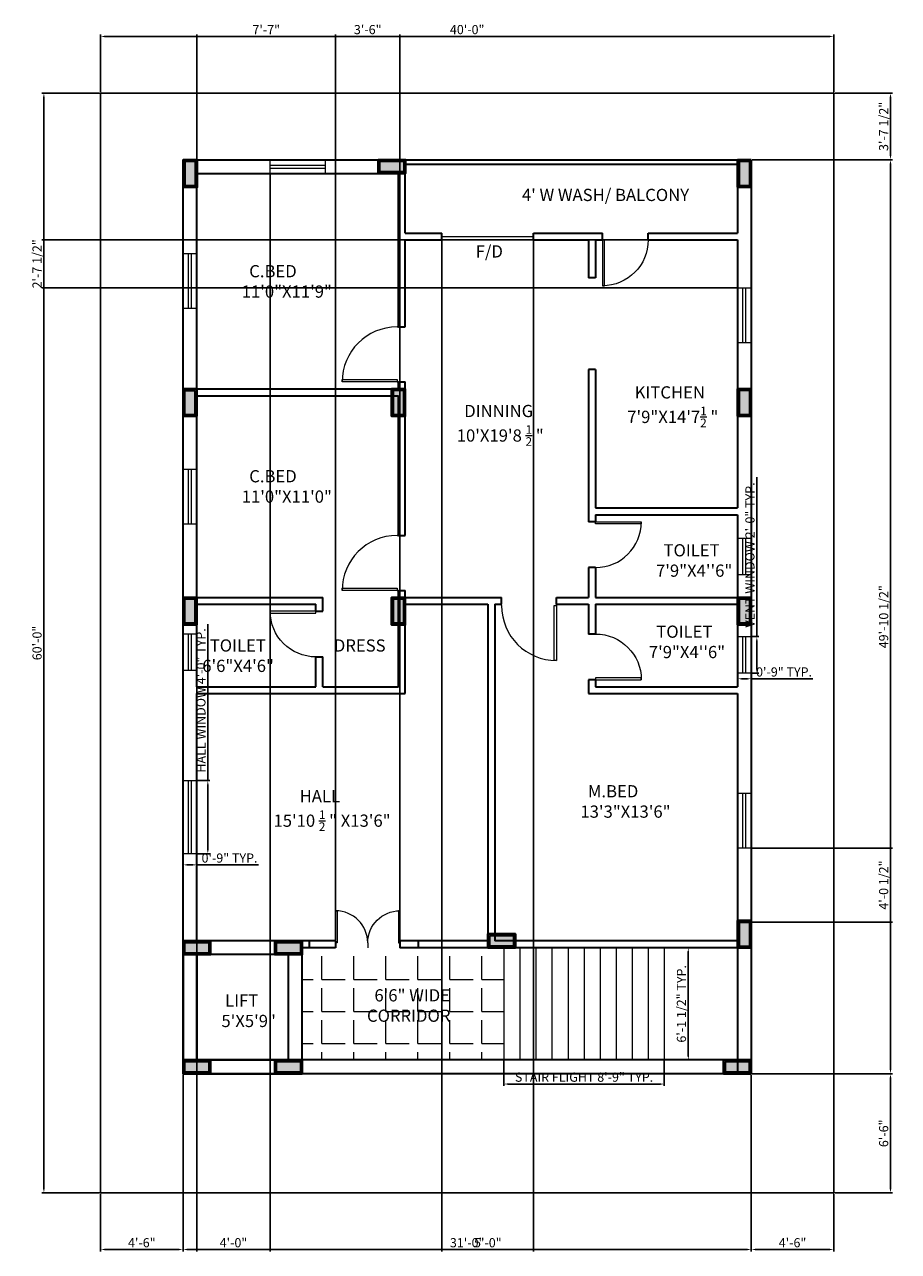
# Model space of a CAD drawing. Units: inches. Extents: x 1678 to 4856, y 4 to 3876.
# Tile 4 of 4: x 4284 to 4856, y 3070 to 3873. Entities that reach past the tile are written whole.
import ezdxf

# ---------------------------------------------------------------- set-up
doc = ezdxf.new("R2010")
doc.units = ezdxf.units.IN
for name, color, linetype, lineweight in [('A-ANNO-TEXT', 7, 'Continuous', 18), ('A-AREA-IDEN', 7, 'Continuous', 18), ('A-FLOR-EVTR', 7, 'Continuous', 35), ('A-FLOR-PATT', 252, 'Continuous', 13), ('COL', 6, 'Continuous', 40), ('compound wall', 7, 'Continuous', 30), ('DIMENSIONS', 6, 'Continuous', 18), ('doors', 2, 'Continuous', 18), ('stairs', 1, 'Continuous', 18), ('walls', 7, 'Continuous', 35), ('windows', 4, 'Continuous', 18)]:
    doc.layers.add(name, color=color, linetype=linetype, lineweight=lineweight)
doc.styles.get("Standard").update_dxf_attribs({"font": 'arial.ttf'})
doc.dimstyles.new('ISO-25', dxfattribs={"dimtxt": 6, "dimasz": 2.5, "dimexe": 1.25, "dimexo": 0.625, "dimtad": 1, "dimdec": 1, "dimlunit": 4, "dimtxsty": 'Standard', "dimcen": 2.5, "dimadec": 0, "dimazin": 0, "dimtfac": 1, "dimtdec": 1, "dimtmove": 0, "dimatfit": 3, "dimfxl": 1, "dimarcsym": 0})

# ---------------------------------------------------------------- blocks, each defined once
blk = doc.blocks.new('*U2')
for p, q in [((0, 0), (0, -6)), ((40, 0), (40, -6))]:
    blk.add_line(p, q)
blk.add_lwpolyline([(0, 0), (0, 40), (1.75, 40), (1.75, 0)], close=True)
blk.add_arc((0, 0), 40, 0, 90)
blk = doc.blocks.new('COLUMN-9x18')
h = blk.add_hatch(color=256)
h.dxf.hatch_style = 1
h.paths.add_polyline_path([(8, 1), (8, 17), (1, 17), (1, 1)])
for points in [[(9, 18), (9, 0), (0, 0), (0, 18)], [(8, 17), (8, 1), (1, 1), (1, 17)]]:
    blk.add_lwpolyline(points, close=True)
blk = doc.blocks.new('WIN-36')
for p, q in [((3.5, 0), (3.5, 36)), ((5.5, 0), (5.5, 36))]:
    blk.add_line(p, q)
blk.add_lwpolyline([(0, 0), (0, 36), (9, 36), (9, 0)], close=True)
blk = doc.blocks.new('WIN-24')
for p, q in [((3.5, 0), (3.5, 24)), ((5.5, 0), (5.5, 24))]:
    blk.add_line(p, q)
blk.add_lwpolyline([(0, 0), (0, 24), (9, 24), (9, 0)], close=True)
blk = doc.blocks.new('WIN-48')
for p, q in [((3.5, 0), (3.5, 48)), ((5.5, 0), (5.5, 48))]:
    blk.add_line(p, q)
blk.add_lwpolyline([(0, 0), (0, 48), (9, 48), (9, 0)], close=True)
blk = doc.blocks.new('SITE-PERIMETER-40x60')
for p, q in [((0, 720), (480, 720)), ((0, 0), (0, 720)), ((480, 720), (480, 0)), ((480, 0), (0, 0))]:
    blk.add_line(p, q)
blk = doc.blocks.new('STAIR-FLIGHT-11-TREAD-LINES')
for p, q in [((0, 73.5), (0, 0)), ((10.5, 73.5), (10.5, 0)), ((21, 73.5), (21, 0)), ((31.5, 73.5), (31.5, 0)), ((42, 73.5), (42, 0)), ((52.5, 73.5), (52.5, 0)), ((63, 73.5), (63, 0)), ((73.5, 73.5), (73.5, 0)), ((84, 73.5), (84, 0)), ((94.5, 73.5), (94.5, 0)), ((105, 73.5), (105, 0))]:
    blk.add_line(p, q)
blk = doc.blocks.new('LIFT-SHAFT-60x69')
for p, q in [((9, 9), (9, 78)), ((69, 9), (9, 9))]:
    blk.add_line(p, q)
blk.add_lwpolyline([(78, 87), (78, 87), (0, 87), (0, 0), (78, 0), (78, 82.5)])
blk.add_lwpolyline([(9, 9), (69, 9), (69, 78), (9, 78)], close=True)
blk = doc.blocks.new('*D46')
at = {"layer": 'Defpoints', "color": 0, "transparency": 16777216}
for p in [(4598, 3195.28), (4703, 3195.28), (4703, 3179.53)]:
    blk.add_point(p, dxfattribs=at)
at = {"layer": 'DIMENSIONS', "color": 0, "lineweight": -2, "transparency": 16777216}
for p, q in [((4598, 3194.65), (4598, 3178.28)), ((4703, 3194.65), (4703, 3178.28)), ((4600.5, 3179.53), (4700.5, 3179.53))]:
    blk.add_line(p, q, dxfattribs=at)
at = {"layer": 'DIMENSIONS', "color": 0, "transparency": 16777216}
for points in [[(4600.5, 3179.94), (4600.5, 3179.11), (4598, 3179.53)], [(4700.5, 3179.94), (4700.5, 3179.11), (4703, 3179.53)]]:
    blk.add_solid(points, dxfattribs=at)
at = {"layer": 'DIMENSIONS', "color": 0, "transparency": 16777216, "insert": (4650.5, 3183.25), "char_height": 6, "attachment_point": 5}
blk.add_mtext('STAIR FLIGHT 8\'-9" TYP.', dxfattribs=at)
blk = doc.blocks.new('*D47')
at = {"layer": 'Defpoints', "color": 0, "transparency": 16777216}
for p in [(4703, 3268.78), (4718.75, 3268.78), (4703, 3195.28)]:
    blk.add_point(p, dxfattribs=at)
at = {"layer": 'DIMENSIONS', "color": 0, "lineweight": -2, "transparency": 16777216}
for p, q in [((4703.63, 3268.78), (4720, 3268.78)), ((4718.75, 3197.78), (4718.75, 3266.28)), ((4703.63, 3195.28), (4720, 3195.28))]:
    blk.add_line(p, q, dxfattribs=at)
at = {"layer": 'DIMENSIONS', "color": 0, "transparency": 16777216}
for points in [[(4718.34, 3266.28), (4719.17, 3266.28), (4718.75, 3268.78)], [(4718.34, 3197.78), (4719.17, 3197.78), (4718.75, 3195.28)]]:
    blk.add_solid(points, dxfattribs=at)
at = {"layer": 'DIMENSIONS', "color": 0, "transparency": 16777216, "insert": (4715.03, 3232.03), "char_height": 6, "attachment_point": 5, "rotation": 90}
blk.add_mtext('6\'-1 1/2" TYP.', dxfattribs=at)
blk = doc.blocks.new('*D50')
at = {"layer": 'Defpoints', "color": 0, "transparency": 16777216}
for p in [(4760, 3472.44), (4763.6, 3472.44), (4760, 3448.44)]:
    blk.add_point(p, dxfattribs=at)
at = {"layer": 'DIMENSIONS', "color": 0, "lineweight": -2, "transparency": 16777216}
for p, q in [((4763.6, 3472.44), (4763.6, 3576.86)), ((4760.63, 3472.44), (4764.85, 3472.44)), ((4763.6, 3450.94), (4763.6, 3469.94)), ((4760.63, 3448.44), (4764.85, 3448.44))]:
    blk.add_line(p, q, dxfattribs=at)
at = {"layer": 'DIMENSIONS', "color": 0, "transparency": 16777216}
for points in [[(4763.19, 3469.94), (4764.02, 3469.94), (4763.6, 3472.44)], [(4763.19, 3450.94), (4764.02, 3450.94), (4763.6, 3448.44)]]:
    blk.add_solid(points, dxfattribs=at)
at = {"layer": 'DIMENSIONS', "color": 0, "transparency": 16777216, "insert": (4759.88, 3525.9), "char_height": 6, "attachment_point": 5, "rotation": 90}
blk.add_mtext('VENT WINDOW 2\'-0" TYP.', dxfattribs=at)
blk = doc.blocks.new('*D51')
at = {"layer": 'Defpoints', "color": 0, "transparency": 16777216}
for p in [(4751, 3448.44), (4760, 3448.44), (4760, 3444.84)]:
    blk.add_point(p, dxfattribs=at)
at = {"layer": 'DIMENSIONS', "color": 0, "lineweight": -2, "transparency": 16777216}
for p, q in [((4751, 3447.82), (4751, 3443.59)), ((4760, 3447.82), (4760, 3443.59)), ((4753.5, 3444.84), (4757.5, 3444.84)), ((4760, 3444.84), (4800.33, 3444.84))]:
    blk.add_line(p, q, dxfattribs=at)
at = {"layer": 'DIMENSIONS', "color": 0, "transparency": 16777216}
for points in [[(4753.5, 3445.26), (4753.5, 3444.42), (4751, 3444.84)], [(4757.5, 3445.26), (4757.5, 3444.42), (4760, 3444.84)]]:
    blk.add_solid(points, dxfattribs=at)
at = {"layer": 'DIMENSIONS', "color": 0, "transparency": 16777216, "insert": (4781.42, 3448.53), "char_height": 6, "attachment_point": 5}
blk.add_mtext('0\'-9" TYP.', dxfattribs=at)
blk = doc.blocks.new('*D52')
at = {"layer": 'Defpoints', "color": 0, "transparency": 16777216}
for p in [(4397, 3378.22), (4404.2, 3378.22), (4397, 3330.22)]:
    blk.add_point(p, dxfattribs=at)
at = {"layer": 'DIMENSIONS', "color": 0, "lineweight": -2, "transparency": 16777216}
for p, q in [((4404.2, 3378.22), (4404.2, 3480.62)), ((4397.63, 3378.22), (4405.45, 3378.22)), ((4404.2, 3332.72), (4404.2, 3375.72)), ((4397.63, 3330.22), (4405.45, 3330.22))]:
    blk.add_line(p, q, dxfattribs=at)
at = {"layer": 'DIMENSIONS', "color": 0, "transparency": 16777216}
for points in [[(4403.79, 3375.72), (4404.62, 3375.72), (4404.2, 3378.22)], [(4403.79, 3332.72), (4404.62, 3332.72), (4404.2, 3330.22)]]:
    blk.add_solid(points, dxfattribs=at)
at = {"layer": 'DIMENSIONS', "color": 0, "transparency": 16777216, "insert": (4400.48, 3430.67), "char_height": 6, "attachment_point": 5, "rotation": 90}
blk.add_mtext('HALL WINDOW 4\'-0" TYP.', dxfattribs=at)
blk = doc.blocks.new('*D53')
at = {"layer": 'Defpoints', "color": 0, "transparency": 16777216}
for p in [(4388, 3330.22), (4397, 3330.22), (4397, 3323.02)]:
    blk.add_point(p, dxfattribs=at)
at = {"layer": 'DIMENSIONS', "color": 0, "lineweight": -2, "transparency": 16777216}
for p, q in [((4388, 3329.6), (4388, 3321.77)), ((4397, 3329.6), (4397, 3321.77)), ((4390.5, 3323.02), (4394.5, 3323.02)), ((4397, 3323.02), (4437.33, 3323.02))]:
    blk.add_line(p, q, dxfattribs=at)
at = {"layer": 'DIMENSIONS', "color": 0, "transparency": 16777216}
for points in [[(4390.5, 3323.44), (4390.5, 3322.6), (4388, 3323.02)], [(4394.5, 3323.44), (4394.5, 3322.6), (4397, 3323.02)]]:
    blk.add_solid(points, dxfattribs=at)
at = {"layer": 'DIMENSIONS', "color": 0, "transparency": 16777216, "insert": (4418.42, 3326.71), "char_height": 6, "attachment_point": 5}
blk.add_mtext('0\'-9" TYP.', dxfattribs=at)
blk = doc.blocks.new('*D62')
at = {"layer": 'Defpoints', "color": 0, "transparency": 16777216}
for p in [(4814, 3865.38), (4334, 3828.28), (4814, 3828.28)]:
    blk.add_point(p, dxfattribs=at)
at = {"layer": 'DIMENSIONS', "color": 0, "lineweight": -2, "transparency": 16777216}
for p, q in [((4334, 3828.9), (4334, 3866.63)), ((4336.5, 3865.38), (4811.5, 3865.38)), ((4814, 3828.9), (4814, 3866.63))]:
    blk.add_line(p, q, dxfattribs=at)
at = {"layer": 'DIMENSIONS', "color": 0, "transparency": 16777216}
for points in [[(4336.5, 3865.79), (4336.5, 3864.96), (4334, 3865.38)], [(4811.5, 3865.79), (4811.5, 3864.96), (4814, 3865.38)]]:
    blk.add_solid(points, dxfattribs=at)
at = {"layer": 'DIMENSIONS', "color": 0, "transparency": 16777216, "insert": (4574, 3869.07), "char_height": 6, "attachment_point": 5}
blk.add_mtext('40\'-0"', dxfattribs=at)
blk = doc.blocks.new('*D63')
at = {"layer": 'Defpoints', "color": 0, "transparency": 16777216}
for p in [(4296.9, 3828.28), (4334, 3828.28), (4334, 3108.28)]:
    blk.add_point(p, dxfattribs=at)
at = {"layer": 'DIMENSIONS', "color": 0, "lineweight": -2, "transparency": 16777216}
for p, q in [((4333.38, 3828.28), (4295.65, 3828.28)), ((4296.9, 3110.78), (4296.9, 3825.78)), ((4333.38, 3108.28), (4295.65, 3108.28))]:
    blk.add_line(p, q, dxfattribs=at)
at = {"layer": 'DIMENSIONS', "color": 0, "transparency": 16777216}
for points in [[(4296.49, 3825.78), (4297.32, 3825.78), (4296.9, 3828.28)], [(4296.49, 3110.78), (4297.32, 3110.78), (4296.9, 3108.28)]]:
    blk.add_solid(points, dxfattribs=at)
at = {"layer": 'DIMENSIONS', "color": 0, "transparency": 16777216, "insert": (4293.22, 3468.28), "char_height": 6, "attachment_point": 5, "rotation": 90}
blk.add_mtext('60\'-0"', dxfattribs=at)
blk = doc.blocks.new('*D64')
at = {"layer": 'Defpoints', "color": 0, "transparency": 16777216}
for p in [(4388, 3186.28), (4760, 3186.28), (4760, 3071.18)]:
    blk.add_point(p, dxfattribs=at)
at = {"layer": 'DIMENSIONS', "color": 0, "lineweight": -2, "transparency": 16777216}
for p, q in [((4388, 3185.65), (4388, 3069.93)), ((4760, 3185.65), (4760, 3069.93)), ((4390.5, 3071.18), (4757.5, 3071.18))]:
    blk.add_line(p, q, dxfattribs=at)
at = {"layer": 'DIMENSIONS', "color": 0, "transparency": 16777216}
for points in [[(4390.5, 3071.59), (4390.5, 3070.76), (4388, 3071.18)], [(4757.5, 3071.59), (4757.5, 3070.76), (4760, 3071.18)]]:
    blk.add_solid(points, dxfattribs=at)
at = {"layer": 'DIMENSIONS', "color": 0, "transparency": 16777216, "insert": (4574, 3074.87), "char_height": 6, "attachment_point": 5}
blk.add_mtext('31\'-0"', dxfattribs=at)
blk = doc.blocks.new('*D65')
at = {"layer": 'Defpoints', "color": 0, "transparency": 16777216}
for p in [(4760, 3784.66), (4851.1, 3784.66), (4760, 3186.28)]:
    blk.add_point(p, dxfattribs=at)
at = {"layer": 'DIMENSIONS', "color": 0, "lineweight": -2, "transparency": 16777216}
for p, q in [((4760.63, 3784.66), (4852.35, 3784.66)), ((4851.1, 3188.78), (4851.1, 3782.16)), ((4760.63, 3186.28), (4852.35, 3186.28))]:
    blk.add_line(p, q, dxfattribs=at)
at = {"layer": 'DIMENSIONS', "color": 0, "transparency": 16777216}
for points in [[(4850.69, 3782.16), (4851.52, 3782.16), (4851.1, 3784.66)], [(4850.69, 3188.78), (4851.52, 3188.78), (4851.1, 3186.28)]]:
    blk.add_solid(points, dxfattribs=at)
at = {"layer": 'DIMENSIONS', "color": 0, "transparency": 16777216, "insert": (4847.38, 3485.47), "char_height": 6, "attachment_point": 5, "rotation": 90}
blk.add_mtext('49\'-10 1/2"', dxfattribs=at)
blk = doc.blocks.new('*D66')
at = {"layer": 'Defpoints', "color": 0, "transparency": 16777216}
for p in [(4388, 3186.28), (4334, 3108.28), (4388, 3071.18)]:
    blk.add_point(p, dxfattribs=at)
at = {"layer": 'DIMENSIONS', "color": 0, "lineweight": -2, "transparency": 16777216}
for p, q in [((4388, 3185.65), (4388, 3069.93)), ((4334, 3107.65), (4334, 3069.93)), ((4336.5, 3071.18), (4385.5, 3071.18))]:
    blk.add_line(p, q, dxfattribs=at)
at = {"layer": 'DIMENSIONS', "color": 0, "transparency": 16777216}
for points in [[(4336.5, 3071.59), (4336.5, 3070.76), (4334, 3071.18)], [(4385.5, 3071.59), (4385.5, 3070.76), (4388, 3071.18)]]:
    blk.add_solid(points, dxfattribs=at)
at = {"layer": 'DIMENSIONS', "color": 0, "transparency": 16777216, "insert": (4361, 3074.87), "char_height": 6, "attachment_point": 5}
blk.add_mtext('4\'-6"', dxfattribs=at)
blk = doc.blocks.new('*D67')
at = {"layer": 'Defpoints', "color": 0, "transparency": 16777216}
for p in [(4760, 3186.28), (4814, 3108.28), (4851.1, 3108.28)]:
    blk.add_point(p, dxfattribs=at)
at = {"layer": 'DIMENSIONS', "color": 0, "lineweight": -2, "transparency": 16777216}
for p, q in [((4760.63, 3186.28), (4852.35, 3186.28)), ((4851.1, 3183.78), (4851.1, 3110.78)), ((4814.63, 3108.28), (4852.35, 3108.28))]:
    blk.add_line(p, q, dxfattribs=at)
at = {"layer": 'DIMENSIONS', "color": 0, "transparency": 16777216}
for points in [[(4850.69, 3183.78), (4851.52, 3183.78), (4851.1, 3186.28)], [(4850.69, 3110.78), (4851.52, 3110.78), (4851.1, 3108.28)]]:
    blk.add_solid(points, dxfattribs=at)
at = {"layer": 'DIMENSIONS', "color": 0, "transparency": 16777216, "insert": (4847.42, 3147.28), "char_height": 6, "attachment_point": 5, "rotation": 90}
blk.add_mtext('6\'-6"', dxfattribs=at)
blk = doc.blocks.new('*D68')
at = {"layer": 'Defpoints', "color": 0, "transparency": 16777216}
for p in [(4814, 3828.28), (4851.1, 3828.28), (4760, 3784.66)]:
    blk.add_point(p, dxfattribs=at)
at = {"layer": 'DIMENSIONS', "color": 0, "lineweight": -2, "transparency": 16777216}
for p, q in [((4814.63, 3828.28), (4852.35, 3828.28)), ((4851.1, 3787.16), (4851.1, 3825.78)), ((4760.63, 3784.66), (4852.35, 3784.66))]:
    blk.add_line(p, q, dxfattribs=at)
at = {"layer": 'DIMENSIONS', "color": 0, "transparency": 16777216}
for points in [[(4850.69, 3825.78), (4851.52, 3825.78), (4851.1, 3828.28)], [(4850.69, 3787.16), (4851.52, 3787.16), (4851.1, 3784.66)]]:
    blk.add_solid(points, dxfattribs=at)
at = {"layer": 'DIMENSIONS', "color": 0, "transparency": 16777216, "insert": (4847.38, 3806.47), "char_height": 6, "attachment_point": 5, "rotation": 90}
blk.add_mtext('3\'-7 1/2"', dxfattribs=at)
blk = doc.blocks.new('*D69')
at = {"layer": 'Defpoints', "color": 0, "transparency": 16777216}
for p in [(4760, 3186.28), (4814, 3108.28), (4814, 3071.18)]:
    blk.add_point(p, dxfattribs=at)
at = {"layer": 'DIMENSIONS', "color": 0, "lineweight": -2, "transparency": 16777216}
for p, q in [((4760, 3185.65), (4760, 3069.93)), ((4814, 3107.65), (4814, 3069.93)), ((4762.5, 3071.18), (4811.5, 3071.18))]:
    blk.add_line(p, q, dxfattribs=at)
at = {"layer": 'DIMENSIONS', "color": 0, "transparency": 16777216}
for points in [[(4762.5, 3071.59), (4762.5, 3070.76), (4760, 3071.18)], [(4811.5, 3071.59), (4811.5, 3070.76), (4814, 3071.18)]]:
    blk.add_solid(points, dxfattribs=at)
at = {"layer": 'DIMENSIONS', "color": 0, "transparency": 16777216, "insert": (4787, 3074.87), "char_height": 6, "attachment_point": 5}
blk.add_mtext('4\'-6"', dxfattribs=at)
blk = doc.blocks.new('*D70')
at = {"layer": 'Defpoints', "color": 0, "transparency": 16777216}
for p in [(4397, 3775.66), (4445, 3775.66), (4445, 3071.18)]:
    blk.add_point(p, dxfattribs=at)
at = {"layer": 'DIMENSIONS', "color": 0, "lineweight": -2, "transparency": 16777216}
for p, q in [((4397, 3775.04), (4397, 3069.93)), ((4445, 3775.04), (4445, 3069.93)), ((4399.5, 3071.18), (4442.5, 3071.18))]:
    blk.add_line(p, q, dxfattribs=at)
at = {"layer": 'DIMENSIONS', "color": 0, "transparency": 16777216}
for points in [[(4399.5, 3071.59), (4399.5, 3070.76), (4397, 3071.18)], [(4442.5, 3071.59), (4442.5, 3070.76), (4445, 3071.18)]]:
    blk.add_solid(points, dxfattribs=at)
at = {"layer": 'DIMENSIONS', "color": 0, "transparency": 16777216, "insert": (4421, 3074.87), "char_height": 6, "attachment_point": 5}
blk.add_mtext('4\'-0"', dxfattribs=at)
blk = doc.blocks.new('*D71')
at = {"layer": 'Defpoints', "color": 0, "transparency": 16777216}
for p in [(4557.5, 3736.66), (4617.5, 3736.66), (4617.5, 3071.18)]:
    blk.add_point(p, dxfattribs=at)
at = {"layer": 'DIMENSIONS', "color": 0, "lineweight": -2, "transparency": 16777216}
for p, q in [((4557.5, 3736.04), (4557.5, 3069.93)), ((4617.5, 3736.04), (4617.5, 3069.93)), ((4560, 3071.18), (4615, 3071.18))]:
    blk.add_line(p, q, dxfattribs=at)
at = {"layer": 'DIMENSIONS', "color": 0, "transparency": 16777216}
for points in [[(4560, 3071.59), (4560, 3070.76), (4557.5, 3071.18)], [(4615, 3071.59), (4615, 3070.76), (4617.5, 3071.18)]]:
    blk.add_solid(points, dxfattribs=at)
at = {"layer": 'DIMENSIONS', "color": 0, "transparency": 16777216, "insert": (4587.5, 3074.87), "char_height": 6, "attachment_point": 5}
blk.add_mtext('5\'-0"', dxfattribs=at)
blk = doc.blocks.new('*D72')
at = {"layer": 'Defpoints', "color": 0, "transparency": 16777216}
for p in [(4487.89, 3865.38), (4397, 3273.28), (4487.89, 3273.28)]:
    blk.add_point(p, dxfattribs=at)
at = {"layer": 'DIMENSIONS', "color": 0, "lineweight": -2, "transparency": 16777216}
for p, q in [((4397, 3273.9), (4397, 3866.63)), ((4399.5, 3865.38), (4485.39, 3865.38)), ((4487.89, 3273.9), (4487.89, 3866.63))]:
    blk.add_line(p, q, dxfattribs=at)
at = {"layer": 'DIMENSIONS', "color": 0, "transparency": 16777216}
for points in [[(4399.5, 3865.79), (4399.5, 3864.96), (4397, 3865.38)], [(4485.39, 3865.79), (4485.39, 3864.96), (4487.89, 3865.38)]]:
    blk.add_solid(points, dxfattribs=at)
at = {"layer": 'DIMENSIONS', "color": 0, "transparency": 16777216, "insert": (4442.45, 3869), "char_height": 6, "attachment_point": 5}
blk.add_mtext('7\'-7"', dxfattribs=at)
blk = doc.blocks.new('*D73')
at = {"layer": 'Defpoints', "color": 0, "transparency": 16777216}
for p in [(4529.89, 3865.38), (4487.89, 3273.28), (4529.89, 3273.28)]:
    blk.add_point(p, dxfattribs=at)
at = {"layer": 'DIMENSIONS', "color": 0, "lineweight": -2, "transparency": 16777216}
for p, q in [((4487.89, 3273.9), (4487.89, 3866.63)), ((4490.39, 3865.38), (4527.39, 3865.38)), ((4529.89, 3273.9), (4529.89, 3866.63))]:
    blk.add_line(p, q, dxfattribs=at)
at = {"layer": 'DIMENSIONS', "color": 0, "transparency": 16777216}
for points in [[(4490.39, 3865.79), (4490.39, 3864.96), (4487.89, 3865.38)], [(4527.39, 3865.79), (4527.39, 3864.96), (4529.89, 3865.38)]]:
    blk.add_solid(points, dxfattribs=at)
at = {"layer": 'DIMENSIONS', "color": 0, "transparency": 16777216, "insert": (4508.89, 3869.07), "char_height": 6, "attachment_point": 5}
blk.add_mtext('3\'-6"', dxfattribs=at)
blk = doc.blocks.new('*D80')
at = {"layer": 'Defpoints', "color": 0, "transparency": 16777216}
for p in [(4751, 3732.16), (4296.9, 3700.81), (4751, 3700.81)]:
    blk.add_point(p, dxfattribs=at)
at = {"layer": 'DIMENSIONS', "color": 0, "lineweight": -2, "transparency": 16777216}
for p, q in [((4750.38, 3732.16), (4295.65, 3732.16)), ((4296.9, 3729.66), (4296.9, 3703.31)), ((4750.38, 3700.81), (4295.65, 3700.81))]:
    blk.add_line(p, q, dxfattribs=at)
at = {"layer": 'DIMENSIONS', "color": 0, "transparency": 16777216}
for points in [[(4296.49, 3729.66), (4297.32, 3729.66), (4296.9, 3732.16)], [(4296.49, 3703.31), (4297.32, 3703.31), (4296.9, 3700.81)]]:
    blk.add_solid(points, dxfattribs=at)
at = {"layer": 'DIMENSIONS', "color": 0, "transparency": 16777216, "insert": (4293.18, 3716.49), "char_height": 6, "attachment_point": 5, "rotation": 90}
blk.add_mtext('2\'-7 1/2"', dxfattribs=at)
blk = doc.blocks.new('*D81')
at = {"layer": 'Defpoints', "color": 0, "transparency": 16777216}
for p in [(4760, 3333.97), (4759, 3285.61), (4851.1, 3285.61)]:
    blk.add_point(p, dxfattribs=at)
at = {"layer": 'DIMENSIONS', "color": 0, "lineweight": -2, "transparency": 16777216}
for p, q in [((4760.63, 3333.97), (4852.35, 3333.97)), ((4851.1, 3331.47), (4851.1, 3288.11)), ((4759.63, 3285.61), (4852.35, 3285.61))]:
    blk.add_line(p, q, dxfattribs=at)
at = {"layer": 'DIMENSIONS', "color": 0, "transparency": 16777216}
for points in [[(4850.69, 3331.47), (4851.52, 3331.47), (4851.1, 3333.97)], [(4850.69, 3288.11), (4851.52, 3288.11), (4851.1, 3285.61)]]:
    blk.add_solid(points, dxfattribs=at)
at = {"layer": 'DIMENSIONS', "color": 0, "transparency": 16777216, "insert": (4847.38, 3309.79), "char_height": 6, "attachment_point": 5, "rotation": 90}
blk.add_mtext('4\'-0 1/2"', dxfattribs=at)

msp = doc.modelspace()

# ---------------------------------------------------------------- hatches: boundary and pattern name
at = {"layer": 'A-FLOR-PATT'}
h = msp.add_hatch(dxfattribs=at)
h.set_pattern_fill('ANGLE', color=256, scale=3)
h.set_pattern_definition([(0, (2760.532, 0), (0, 20.955), [15.24, -5.715]), (90, (2760.532, 0), (-20.955, 1e-15), [15.24, -5.715])])
h.paths.add_polyline_path([(4598, 3268.78), (4466, 3268.78), (4466, 3195.28), (4598, 3195.28)])

# ---------------------------------------------------------------- linework, layer by layer
at = {"layer": 'doors'}
msp.add_line((4557.5, 3734.41), (4617.5, 3734.41), dxfattribs=at)
at = {"layer": 'walls'}
for p, q in [((4388, 3784.66), (4760, 3784.66)), ((4388, 3186.28), (4388, 3784.66)), ((4760, 3784.66), (4760, 3186.28)), ((4397, 3775.66), (4529, 3775.66)), ((4397, 3634.66), (4397, 3775.66)), ((4529, 3675.16), (4529, 3775.66)), ((4533.5, 3781.66), (4751, 3781.66)), ((4533.5, 3736.66), (4533.5, 3781.66)), ((4751, 3781.66), (4751, 3736.66)), ((4533.5, 3736.66), (4557.5, 3736.66)), ((4557.5, 3732.16), (4557.5, 3736.66)), ((4617.5, 3736.66), (4662.5, 3736.66)), ((4617.5, 3732.16), (4617.5, 3736.66)), ((4662.5, 3732.16), (4662.5, 3736.66)), ((4692.5, 3736.66), (4751, 3736.66)), ((4692.5, 3732.16), (4692.5, 3736.66)), ((4533.5, 3732.16), (4557.5, 3732.16)), ((4533.5, 3675.16), (4533.5, 3732.16)), ((4617.5, 3732.16), (4653.5, 3732.16)), ((4653.5, 3732.16), (4653.5, 3707.41)), ((4658, 3732.16), (4662.5, 3732.16)), ((4658, 3732.16), (4658, 3707.41)), ((4692.5, 3732.16), (4751, 3732.16)), ((4751, 3732.16), (4751, 3556.66)), ((4658, 3707.41), (4653.5, 3707.41)), ((4529, 3675.16), (4533.5, 3675.16)), ((4653.5, 3647.41), (4653.5, 3547.66)), ((4658, 3647.41), (4653.5, 3647.41)), ((4658, 3647.41), (4658, 3556.66)), ((4529, 3634.66), (4529, 3639.16)), ((4529, 3639.16), (4533.5, 3639.16)), ((4533.5, 3538.66), (4533.5, 3639.16)), ((4397, 3634.66), (4529, 3634.66)), ((4397, 3630.16), (4529, 3630.16)), ((4397, 3498.16), (4397, 3630.16)), ((4529, 3538.66), (4529, 3630.16)), ((4658, 3630.16), (4658, 3556.66)), ((4658, 3556.66), (4751, 3556.66)), ((4658, 3552.16), (4751, 3552.16)), ((4658, 3552.16), (4658, 3547.66)), ((4751, 3552.16), (4751, 3498.16)), ((4658, 3547.66), (4653.5, 3547.66)), ((4529, 3538.66), (4533.5, 3538.66)), ((4653.5, 3517.66), (4653.5, 3498.16)), ((4658, 3517.66), (4653.5, 3517.66)), ((4658, 3517.66), (4658, 3498.16)), ((4529, 3498.16), (4529, 3502.66)), ((4529, 3502.66), (4533.5, 3502.66)), ((4533.5, 3498.16), (4533.5, 3502.66)), ((4397, 3498.16), (4479.5, 3498.16)), ((4479.5, 3489.16), (4479.5, 3498.16)), ((4529, 3439.66), (4529, 3498.16)), ((4533.5, 3498.16), (4596.5, 3498.16)), ((4596.5, 3493.66), (4596.5, 3498.16)), ((4632.5, 3498.16), (4653.5, 3498.16)), ((4632.5, 3493.66), (4632.5, 3498.16)), ((4658, 3498.16), (4751, 3498.16)), ((4397, 3493.66), (4475, 3493.66)), ((4397, 3439.66), (4397, 3493.66)), ((4475, 3489.16), (4475, 3493.66)), ((4475, 3489.16), (4479.5, 3489.16)), ((4479.5, 3489.16), (4479.5, 3489.16)), ((4533.5, 3493.66), (4587.5, 3493.66)), ((4533.5, 3435.16), (4533.5, 3493.66)), ((4587.5, 3493.66), (4587.5, 3273.28)), ((4592, 3493.66), (4596.5, 3493.66)), ((4592, 3493.66), (4592, 3273.28)), ((4632.5, 3493.66), (4653.5, 3493.66)), ((4653.5, 3493.66), (4653.5, 3474.16)), ((4658, 3493.66), (4751, 3493.66)), ((4658, 3493.66), (4658, 3474.16)), ((4751, 3493.66), (4751, 3439.66)), ((4658, 3474.16), (4653.5, 3474.16)), ((4475, 3439.66), (4475, 3459.16)), ((4475, 3459.16), (4479.5, 3459.16)), ((4479.5, 3439.66), (4479.5, 3459.16)), ((4397, 3439.66), (4475, 3439.66)), ((4479.5, 3439.66), (4529, 3439.66)), ((4653.5, 3444.16), (4653.5, 3435.16)), ((4658, 3444.16), (4653.5, 3444.16)), ((4658, 3444.16), (4658, 3439.66)), ((4658, 3439.66), (4751, 3439.66)), ((4397, 3435.16), (4533.5, 3435.16)), ((4397, 3273.28), (4397, 3435.16)), ((4653.5, 3435.16), (4751, 3435.16)), ((4751, 3435.16), (4751, 3268.78)), ((4487.89, 3273.28), (4397, 3273.28)), ((4470.5, 3273.28), (4470.5, 3268.78)), ((4470.5, 3273.28), (4470.5, 3268.78)), ((4487.89, 3273.28), (4487.89, 3268.78)), ((4587.5, 3273.28), (4529.89, 3273.28)), ((4529.89, 3273.28), (4529.89, 3268.78)), ((4541.89, 3273.28), (4541.89, 3268.78)), ((4751, 3273.28), (4592, 3273.28)), ((4487.89, 3268.78), (4466, 3268.78)), ((4751, 3268.78), (4529.89, 3268.78)), ((4751, 3268.78), (4751, 3186.28)), ((4760, 3195.28), (4466, 3195.28)), ((4760, 3186.28), (4388, 3186.28))]:
    msp.add_line(p, q, dxfattribs=at)

# ---------------------------------------------------------------- block references
at = {"layer": 'A-FLOR-EVTR'}
msp.add_blockref('LIFT-SHAFT-60x69', (4388, 3186.28), dxfattribs=at)
at = {"layer": 'COL'}
for p in [(4388.24, 3766.66), (4751, 3766.66), (4388, 3616.66), (4524.5, 3616.69), (4751, 3616.69), (4388, 3480.16), (4524.5, 3480.16), (4751, 3480.16), (4751, 3268.61)]:
    msp.add_blockref('COLUMN-9x18', p, dxfattribs=at)
for p, rotation in [((4533.64, 3775.66), 90.00000000001293), ((4605.55, 3268.78), 90.00000000000875), ((4406, 3264.28), 90.00000000000438), ((4466, 3264.28), 90.00000000000438), ((4406, 3186.28), 90.00000000000438), ((4466, 3186.28), 90.00000000000438), ((4759.81, 3186.28), 90.00000000000644)]:
    msp.add_blockref('COLUMN-9x18', p, dxfattribs=dict(at, rotation=rotation))
at = {"layer": 'compound wall', "rotation": 180}
msp.add_blockref('SITE-PERIMETER-40x60', (4814, 3828.28), dxfattribs=at)
at = {"layer": 'doors'}
for p, xscale, yscale, zscale, rotation in [((4662.5, 3732.16), -0.75, 0.75, 0.75, 180), ((4528.1, 3639.16), 0.9, 0.9, 0.9, 89.99999999999999), ((4658, 3547.66), 0.75, 0.75, 0.75, 270), ((4528.1, 3502.66), 0.9, 0.9, 0.9, 89.99999999999999), ((4632.5, 3492.76), 0.9, 0.9, 0.9, 180), ((4475, 3489.16), -0.75, 0.75, 0.75, 90), ((4658, 3444.16), -0.75, 0.75, 0.75, 270)]:
    msp.add_blockref('*U2', p, dxfattribs=dict(at, xscale=xscale, yscale=yscale, zscale=zscale, rotation=rotation))
at = {"layer": 'doors', "yscale": 0.525, "zscale": 0.525}
for p, xscale in [((4487.89, 3271.93), 0.525), ((4529.89, 3271.93), -0.525)]:
    msp.add_blockref('*U2', p, dxfattribs=dict(at, xscale=xscale))
at = {"layer": 'stairs'}
msp.add_blockref('STAIR-FLIGHT-11-TREAD-LINES', (4598, 3195.28), dxfattribs=at)
at = {"layer": 'windows', "rotation": 270.0000000000033}
msp.add_blockref('WIN-36', (4445, 3784.66), dxfattribs=at)
at = {"layer": 'windows'}
for name, p in [('WIN-36', (4388, 3687.16)), ('WIN-36', (4751, 3664.81)), ('WIN-36', (4388, 3546.16)), ('WIN-24', (4751, 3512.94)), ('WIN-24', (4388, 3450.26)), ('WIN-24', (4751, 3448.44)), ('WIN-48', (4388, 3330.22)), ('WIN-36', (4751, 3333.97))]:
    msp.add_blockref(name, p, dxfattribs=at)

# ---------------------------------------------------------------- texts
at = {"layer": 'A-ANNO-TEXT', "insert": (4579.57, 3728.64), "char_height": 8, "attachment_point": 1}
msp.add_mtext_dynamic_manual_height_columns('F/D', width=15.7651, gutter_width=12.5, heights=[0], dxfattribs=at)
at = {"layer": 'A-AREA-IDEN', "char_height": 8, "attachment_point": 1}
for s, width, insert in [("4' W WASH/ BALCONY", 120.7362, (4609.83, 3765.6)), ('\\pxqj;  C.BED\\P\\pq*;11\'0"X11\'9"', 58.5808, (4426.42, 3715.68)), ('\\A1;  KITCHEN\\P7\'9"X14\'7{\\H0.7x;\\S1/2;} "', 64.7201, (4678.77, 3636.34)), ('\\A1;  DINNING\\P10\'X19\'8 {\\H0.7x;\\S1/2;} "', 64.7201, (4567.18, 3624.15)), ('\\pxqj;  C.BED\\P\\pq*;11\'0"X11\'0"', 58.5808, (4426.42, 3581.44)), ('  TOILET\\P7\'9"X4\'\'6"', 58.5808, (4697.63, 3532.97)), ('  TOILET\\P7\'9"X4\'\'6"', 58.5808, (4692.92, 3479.68)), ('  TOILET\\P6\'6"X4\'6"', 58.5808, (4400.58, 3470.64)), ('  DRESS', 58.5808, (4481.82, 3470.64)), ('\\pxqj;  M.BED\\P\\pq*;13\'3"X13\'6"', 58.5808, (4648.13, 3375.22)), ('\\A1;\\pxqj;       HALL\\P\\pq*;15\'10 {\\H0.7x;\\S1/2;} " X13\'6"', 80.3743, (4447.22, 3372)), (' LIFT\\P5\'X5\'9"', 58.5808, (4413.11, 3238.17)), ('  6\'6" WIDE\\PCORRIDOR', 58.5808, (4508.39, 3241.61))]:
    msp.add_mtext_dynamic_manual_height_columns(s, width=width, gutter_width=12.5, heights=[0], dxfattribs=dict(at, insert=insert))

# ---------------------------------------------------------------- dimensions: what is measured, and where the dimension line sits
at = {"layer": 'DIMENSIONS'}
for base, p1, p2, picture, middle in [((4814, 3865.38), (4334, 3828.28), (4814, 3828.28), '*D62', (4574, 3869.07)), ((4487.89, 3865.38), (4397, 3273.28), (4487.89, 3273.28), '*D72', (4442.45, 3869)), ((4529.89, 3865.38), (4487.89, 3273.28), (4529.89, 3273.28), '*D73', (4508.89, 3869.07)), ((4445, 3071.18), (4397, 3775.66), (4445, 3775.66), '*D70', (4421, 3074.87)), ((4617.5, 3071.18), (4557.5, 3736.66), (4617.5, 3736.66), '*D71', (4587.5, 3074.87)), ((4388, 3071.18), (4334, 3108.28), (4388, 3186.28), '*D66', (4361, 3074.87)), ((4760, 3071.18), (4388, 3186.28), (4760, 3186.28), '*D64', (4574, 3074.87)), ((4814, 3071.18), (4760, 3186.28), (4814, 3108.28), '*D69', (4787, 3074.87))]:
    dim = msp.add_linear_dim(base=base, p1=p1, p2=p2, dimstyle='ISO-25', override={"dimdec": 1, "dimlfac": 1, "dimrnd": 0, "dimzin": 1, "dimdsep": 46, "dimlunit": 4, "dimfrac": 2}, dxfattribs=at)
    dim.commit()
    dim.dimension.update_dxf_attribs({"geometry": picture, "text_midpoint": middle})
for base, p1, p2, picture, middle in [((4296.9, 3828.28), (4334, 3108.28), (4334, 3828.28), '*D63', (4293.22, 3468.28)), ((4851.1, 3828.28), (4760, 3784.66), (4814, 3828.28), '*D68', (4847.38, 3806.47)), ((4851.1, 3784.66), (4760, 3186.28), (4760, 3784.66), '*D65', (4847.38, 3485.47)), ((4296.9046, 3700.8147), (4751.0046, 3732.1642), (4751.0046, 3700.8147), '*D80', (4293.1772, 3716.4894)), ((4851.1, 3285.61), (4760, 3333.97), (4759, 3285.61), '*D81', (4847.38, 3309.79)), ((4851.1, 3108.28), (4760, 3186.28), (4814, 3108.28), '*D67', (4847.42, 3147.28))]:
    dim = msp.add_linear_dim(base=base, p1=p1, p2=p2, angle=90, dimstyle='ISO-25', override={"dimdec": 1, "dimlfac": 1, "dimrnd": 0, "dimzin": 1, "dimdsep": 46, "dimlunit": 4, "dimfrac": 2}, dxfattribs=at)
    dim.commit()
    dim.dimension.update_dxf_attribs({"geometry": picture, "text_midpoint": middle})
for base, p1, p2, text, picture, middle in [((4763.6, 3472.44), (4760, 3448.44), (4760, 3472.44), 'VENT WINDOW <> TYP.', '*D50', (4759.88, 3525.9)), ((4404.2, 3378.22), (4397, 3330.22), (4397, 3378.22), 'HALL WINDOW <> TYP.', '*D52', (4400.48, 3430.67)), ((4718.75, 3268.78), (4703, 3195.28), (4703, 3268.78), '<> TYP.', '*D47', (4715.03, 3232.03))]:
    dim = msp.add_linear_dim(base=base, p1=p1, p2=p2, angle=90, text=text, dimstyle='ISO-25', override={"dimdec": 1, "dimlfac": 1, "dimrnd": 0, "dimzin": 1, "dimdsep": 46, "dimlunit": 4, "dimfrac": 2}, dxfattribs=at)
    dim.commit()
    dim.dimension.update_dxf_attribs({"geometry": picture, "text_midpoint": middle})
for base, p1, p2, text, picture, middle in [((4760, 3444.84), (4751, 3448.44), (4760, 3448.44), '<> TYP.', '*D51', (4781.42, 3448.53)), ((4397, 3323.02), (4388, 3330.22), (4397, 3330.22), '<> TYP.', '*D53', (4418.42, 3326.71)), ((4703, 3179.53), (4598, 3195.28), (4703, 3195.28), 'STAIR FLIGHT <> TYP.', '*D46', (4650.5, 3183.25))]:
    dim = msp.add_linear_dim(base=base, p1=p1, p2=p2, text=text, dimstyle='ISO-25', override={"dimdec": 1, "dimlfac": 1, "dimrnd": 0, "dimzin": 1, "dimdsep": 46, "dimlunit": 4, "dimfrac": 2}, dxfattribs=at)
    dim.commit()
    dim.dimension.update_dxf_attribs({"geometry": picture, "text_midpoint": middle})

doc.saveas('drawing.dxf')
